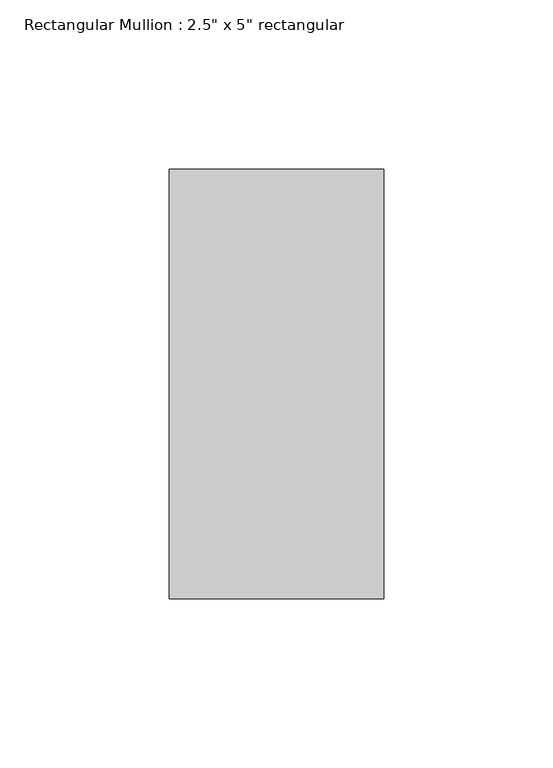
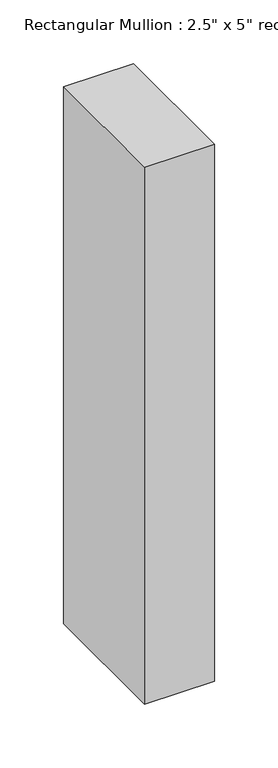
"""IFC4 building model written with IfcOpenShell, lengths in millimetres: member geometry."""

from ifc_helpers import new_model, si_unit, frame, origin, place, context, project, spatial, polyline, outline, extrude, source, transform, mapped, element, save


def member_aaa03826(model_context):
    return source(origin(), model_context, "Body", "SweptSolid", [
        extrude(outline(polyline([(31.75, 63.5), (31.75, -63.5), (-31.75, -63.5), (-31.75, 63.5), (31.75, 63.5)])), frame((0.0, 0.0, -514.35), z_axis=(0.0, 0.0, 1.0), x_axis=(1.0, 0.0, 0.0)), (0.0, 0.0, 1.0), 514.35),
    ])


if __name__ == "__main__":
    model = new_model("IFC4")
    model_context = context("Model", 3, world=origin())
    ifc_project = project(units=[si_unit("LENGTHUNIT", "METRE", prefix="MILLI")], contexts=[model_context])
    site = spatial("IfcSite", under=ifc_project)
    building = spatial("IfcBuilding", under=site)
    placement = place(None, origin())
    member_shape = member_aaa03826(model_context)
    element("IfcMember", 1, ObjectType="Rectangular Mullion : 2.5\" x 5\" rectangular", at=placement, inside=building, context=model_context, shape_type="MappedRepresentation", body=[
        mapped(member_shape, transform((0.0, 0.0, 0.0), x_axis=(1.0, 0.0, 0.0), y_axis=(0.0, 1.0, 0.0), z_axis=(0.0, 0.0, 1.0))),
    ])
    save(model, "model.ifc")

# Revit data of these elements
# Type "Rectangular Mullion : 2.5\" x 5\" rectangular"
#   built-in parameter 1007304 = 0.416667 (stored number, unit not read)
#   built-in parameter 1007301 = 0.104167 (stored number, unit not read)
#   built-in parameter 1007300 = 0.104167 (stored number, unit not read)
